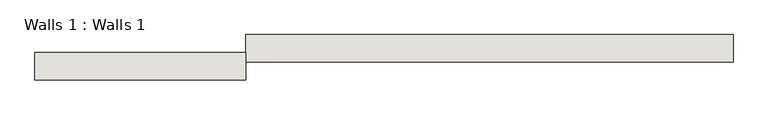
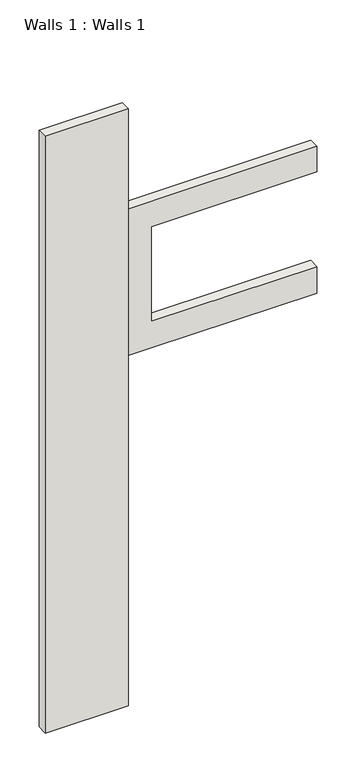
"""IFC4 building model written with IfcOpenShell, lengths in millimetres: wall geometry, Walls 1 : Walls 1."""

from ifc_helpers import new_model, si_unit, frame, origin, place, context, project, spatial, polyline, outline, extrude, source, transform, mapped, element, save


def walls_1_walls_1_998562f7(model_context):
    return source(origin(), model_context, "Body", "SweptSolid", [
        extrude(outline(polyline([(18769.577535, -8856.3304753), (18007.577535, -8856.3304753), (14349.977535, -8856.3304753), (14349.977535, -8094.3304753), (14349.977535, -3369.9304753), (15147.3985306, -3369.9304753), (15147.3985306, -8094.3304753), (18007.577535, -8094.3304753), (18007.577535, -3369.9304753), (18769.577535, -3369.9304753), (18769.577535, -8856.3304753)])), frame((0.0, 2754.0297737, 0.0), z_axis=(0.0, 1.0, 0.0), x_axis=(0.0, 0.0, 1.0)), (0.0, 0.0, 1.0), 304.8),
        extrude(outline(polyline([(-8856.3304753, 2550.8297737), (-11229.7148765, 2550.8297737), (-11229.7148765, 2855.6297737), (-8856.3304753, 2855.6297737), (-8856.3304753, 2550.8297737)])), frame((0.0, 0.0, 3962.4), z_axis=(0.0, 0.0, 1.0), x_axis=(1.0, 0.0, 0.0)), (0.0, 0.0, 1.0), 17983.2),
    ])


if __name__ == "__main__":
    model = new_model("IFC4")
    model_context = context("Model", 3, world=origin())
    ifc_project = project(units=[si_unit("LENGTHUNIT", "METRE", prefix="MILLI")], contexts=[model_context])
    site = spatial("IfcSite", under=ifc_project)
    building = spatial("IfcBuilding", under=site)
    placement = place(None, origin())
    walls_1_walls_1_shape = walls_1_walls_1_998562f7(model_context)
    element("IfcWall", 1, ObjectType="Walls 1 : Walls 1", at=placement, inside=building, context=model_context, shape_type="MappedRepresentation", body=[
        mapped(walls_1_walls_1_shape, transform((0.0, 0.0, 0.0), x_axis=(1.0, 0.0, 0.0), y_axis=(0.0, 1.0, 0.0), z_axis=(0.0, 0.0, 1.0))),
    ])
    save(model, "model.ifc")

# Revit data of these elements
# Element 1 (IfcWall, "Walls 1 : Walls 1")
#   Materials on its faces: "Default Wall"
# Materials
#   "Default Wall": colour RGB 128 128 128, transparency 0
